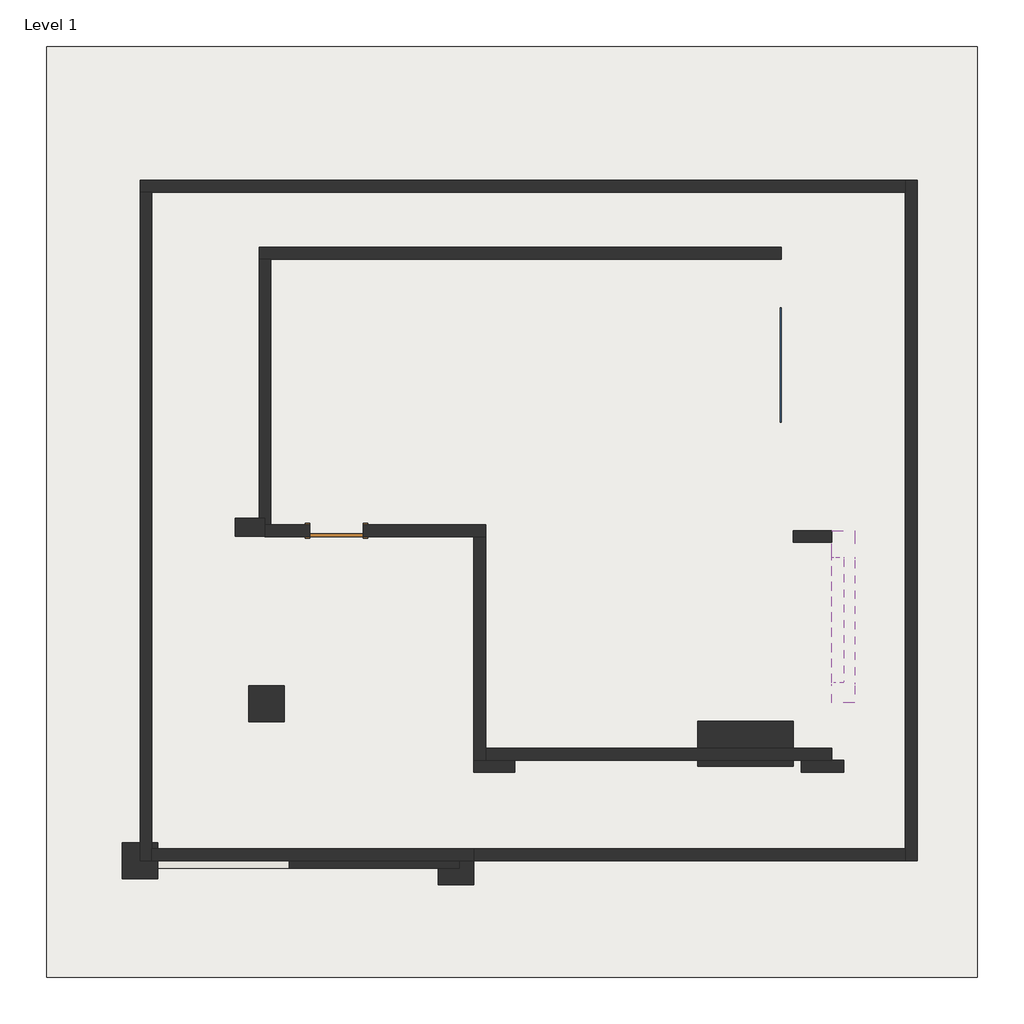
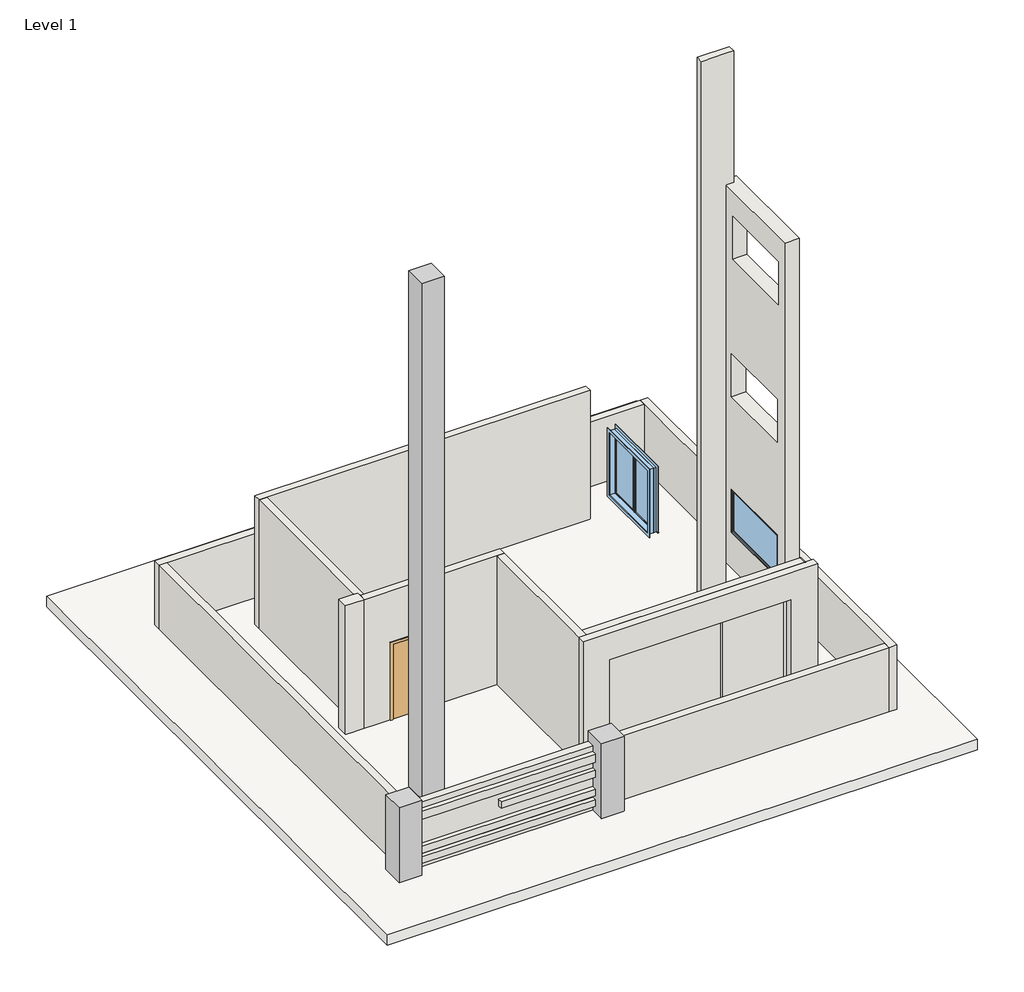
# One storey: 16 walls, 3 columns, 2 windows, 1 door, 1 slab.
"""IFC4 building model written with IfcOpenShell, lengths in millimetres."""

from ifc_helpers import new_model, si_unit, frame, origin, origin_with_axes, place, context, project, spatial, polyline, outline, extrude, faceted_brep, transform, mapped, element, save
from components import column_edfe3d85, door_54dd4da4, walls_2_walls_2_0b909519, walls_3_walls_3_385398a2, walls_4_walls_4_47acbb33, window_b085ff8d, window_a973ac2f

model = new_model("IFC4")

# Units and contexts
model_context = context("Model", 3, world=origin())
ifc_project = project(units=[si_unit("LENGTHUNIT", "METRE", prefix="MILLI")], contexts=[model_context])

# Site, building, storey
site = spatial("IfcSite", under=ifc_project)
building = spatial("IfcBuilding", under=site)
storey = spatial("IfcBuildingStorey", under=building, Name="Level 1", Elevation=0.0)

# Columns
placement = place(None, origin())
element("IfcColumn", 1, ObjectType="Rectangular Column : 24\" x 24\"", at=placement, inside=storey, context=model_context, shape_type="Brep", body=[
    faceted_brep([(-11835.7165692, -1.8724828, 2133.6), (-12445.3165692, -1.8724828, 2133.6), (-12445.3165692, -611.4724828, 2133.6), (-11835.7165692, -611.4724828, 2133.6), (-11937.3165692, -1.8724828, 0.0), (-11835.7165692, -1.8724828, 0.0), (-11835.7165692, -103.4724828, 0.0), (-11937.3165692, -103.4724828, 0.0), (-11937.3165692, -1.8724828, 1828.8), (-12140.5165692, -1.8724828, 1828.8), (-12140.5165692, -1.8724828, 0.0), (-12445.3165692, -1.8724828, 0.0), (-12445.3165692, -611.4724828, 0.0), (-11835.7165692, -611.4724828, 0.0), (-11835.7165692, -306.6724828, 0.0), (-11835.7165692, -306.6724828, 1828.8), (-11835.7165692, -103.4724828, 1828.8), (-11937.3165692, -103.4724828, 1828.8), (-12140.5165692, -306.6724828, 1828.8), (-12140.5165692, -306.6724828, 0.0), (-11937.3165692, -306.6724828, 1828.8), (-11937.3165692, -306.6724828, 0.0)], [[[0, 1, 2, 3]], [[4, 5, 6, 7]], [[1, 0, 5, 4, 8, 9, 10, 11]], [[2, 1, 11, 12]], [[3, 2, 12, 13]], [[0, 3, 13, 14, 15, 16, 6, 5]], [[8, 4, 7, 17]], [[18, 19, 10, 9]], [[20, 18, 9, 8, 17]], [[19, 18, 20, 21]], [[20, 15, 14, 21]], [[16, 17, 7, 6]], [[15, 20, 17, 16]], [[13, 12, 11, 10, 19, 21, 14]]]),
])
element("IfcColumn", 2, ObjectType="Rectangular Column : 24\" x 24\"", at=placement, inside=storey, context=model_context, shape_type="Brep", body=[
    faceted_brep([(-6456.5821198, -102.7094845, 2133.6), (-7066.1821198, -102.7094845, 2133.6), (-7066.1821198, -712.3094845, 2133.6), (-6456.5821198, -712.3094845, 2133.6), (-7066.1821198, -102.7094845, 0.0), (-6456.5821198, -102.7094845, 0.0), (-6456.5821198, -103.4724828, 0.0), (-7066.1821198, -103.4724828, 0.0), (-6456.5821198, -102.7094845, 1828.8), (-7066.1821198, -103.4724828, 1828.8), (-7066.1821198, -306.6724828, 1828.8), (-7066.1821198, -306.6724828, 0.0), (-7066.1821198, -712.3094845, 0.0), (-6456.5821198, -712.3094845, 0.0), (-6456.5821198, -306.6724828, 0.0), (-6456.5821198, -306.6724828, 1828.8), (-6456.5821198, -103.4724828, 1828.8)], [[[0, 1, 2, 3]], [[4, 5, 6, 7]], [[1, 0, 8, 5, 4]], [[2, 1, 4, 7, 9, 10, 11, 12]], [[3, 2, 12, 13]], [[0, 3, 13, 14, 15, 16, 6, 5, 8]], [[10, 15, 14, 11]], [[16, 9, 7, 6]], [[15, 10, 9, 16]], [[13, 12, 11, 14]]]),
])
column_shape = column_edfe3d85(model_context)
element("IfcColumn", 3, ObjectType="Rectangular Column : 24\" x 24\"", at=placement, inside=storey, context=model_context, shape_type="MappedRepresentation", body=[
    mapped(column_shape, transform((-9987.1821198, 2368.60098, 0.0), x_axis=(1.0, 0.0, 0.0), y_axis=(0.0, 1.0, 0.0), z_axis=(0.0, 0.0, 1.0))),
])

# Door
door_shape = door_54dd4da4(model_context)
element("IfcDoor", 4, ObjectType="Single-Flush : 36\" x 84\"", at=placement, inside=storey, context=model_context, shape_type="MappedRepresentation", body=[
    mapped(door_shape, transform((-8793.3821198, 5315.00098, 0.0), x_axis=(-1.0, 0.0, 0.0), y_axis=(0.0, -1.0, 0.0), z_axis=(0.0, 0.0, 1.0))),
])

# Slab
element("IfcSlab", 5, ObjectType="Generic - 12\"", at=placement, inside=storey, context=model_context, shape_type="SweptSolid", body=[
    extrude(outline(polyline([(2117.6840298, 13555.8620749), (2117.6840298, -2293.7379251), (-13731.9159702, -2293.7379251), (-13731.9159702, 13555.8620749), (2117.6840298, 13555.8620749)])), frame((0.0, 0.0, -304.8), z_axis=(0.0, 0.0, 1.0), x_axis=(1.0, 0.0, 0.0)), (0.0, 0.0, 1.0), 304.8),
])

# Walls
element("IfcWall", 6, ObjectType="Generic - 12\"", at=placement, inside=storey, context=model_context, shape_type="Brep", body=[
    faceted_brep([(-10520.5932957, 5216.0652184, 0.0), (-10012.5821198, 5216.0652184, 0.0), (-10012.5821198, 5216.0652184, 3657.6), (-10520.5932957, 5216.0652184, 3657.6), (-10520.5932957, 5520.8652184, 0.0), (-10520.5932957, 5520.8652184, 3657.6), (-10114.1821198, 5520.8652184, 3657.6), (-10012.5821198, 5520.8652184, 3657.6), (-10012.5821198, 5520.8652184, 0.0), (-10114.1821198, 5520.8652184, 0.0), (-10012.5821198, 5416.60098, 0.0), (-10012.5821198, 5416.60098, 3657.6)], [[[0, 1, 2, 3]], [[4, 5, 6, 7, 8, 9]], [[1, 0, 4, 9, 8, 10]], [[2, 1, 10, 8, 7, 11]], [[3, 2, 11, 7, 6, 5]], [[0, 3, 5, 4]]]),
])
element("IfcWall", 7, ObjectType="Generic - 8\"", at=placement, inside=storey, context=model_context, shape_type="Brep", body=[
    faceted_brep([(-10114.1821198, 9937.80098, 0.0), (-9910.9821198, 9937.80098, 0.0), (-1224.1821198, 9937.80098, 0.0), (-1224.1821198, 9937.80098, 3657.6), (-9910.9821198, 9937.80098, 3657.6), (-10114.1821198, 9937.80098, 3657.6), (-10114.1821198, 10141.00098, 0.0), (-10114.1821198, 10141.00098, 3657.6), (-1224.1821198, 10141.00098, 3657.6), (-1224.1821198, 10141.00098, 0.0)], [[[0, 1, 2, 3, 4, 5]], [[6, 7, 8, 9]], [[2, 1, 0, 6, 9]], [[0, 5, 7, 6]], [[5, 4, 3, 8, 7]], [[3, 2, 9, 8]]]),
])
element("IfcWall", 8, ObjectType="Generic - 8\"", at=placement, inside=storey, context=model_context, shape_type="SweptSolid", body=[
    extrude(outline(polyline([(-9910.9821198, 9937.80098), (-9910.9821198, 5416.60098), (-10012.5821198, 5416.60098), (-10012.5821198, 5520.8652184), (-10114.1821198, 5520.8652184), (-10114.1821198, 9937.80098), (-9910.9821198, 9937.80098)])), origin_with_axes(), (0.0, 0.0, 1.0), 3657.6),
])
element("IfcWall", 9, ObjectType="Generic - 8\"", at=placement, inside=storey, context=model_context, shape_type="SweptSolid", body=[
    extrude(outline(polyline([(0.0, -360.5821198), (3657.6, -360.5821198), (3657.6, -385.9821198), (3657.6, -6253.3821198), (0.0, -6253.3821198), (0.0, -360.5821198)])), frame((0.0, 1403.40098, 0.0), z_axis=(0.0, 1.0, 0.0), x_axis=(0.0, 0.0, 1.0)), (0.0, 0.0, 1.0), 203.2),
])
element("IfcWall", 10, ObjectType="Generic - 8\"", at=placement, inside=storey, context=model_context, shape_type="Brep", body=[
    faceted_brep([(-10012.5821198, 5213.40098, 0.0), (-9250.5821198, 5213.40098, 0.0), (-9250.5821198, 5213.40098, 2133.6), (-8336.1821198, 5213.40098, 2133.6), (-8336.1821198, 5213.40098, 0.0), (-6456.5821198, 5213.40098, 0.0), (-6253.3821198, 5213.40098, 0.0), (-6253.3821198, 5213.40098, 3657.6), (-6456.5821198, 5213.40098, 3657.6), (-10012.5821198, 5213.40098, 3657.6), (-9250.5821198, 5416.60098, 2133.6), (-9250.5821198, 5416.60098, 0.0), (-9910.9821198, 5416.60098, 0.0), (-10012.5821198, 5416.60098, 0.0), (-10012.5821198, 5416.60098, 3657.6), (-9910.9821198, 5416.60098, 3657.6), (-6253.3821198, 5416.60098, 3657.6), (-6253.3821198, 5416.60098, 0.0), (-8336.1821198, 5416.60098, 0.0), (-8336.1821198, 5416.60098, 2133.6), (-10012.5821198, 5216.0652184, 0.0), (-10012.5821198, 5216.0652184, 3657.6)], [[[0, 1, 2, 3, 4, 5, 6, 7, 8, 9]], [[10, 11, 12, 13, 14, 15, 16, 17, 18, 19]], [[18, 17, 6, 5, 4]], [[13, 12, 11, 1, 0, 20]], [[9, 8, 7, 16, 15, 14, 21]], [[0, 9, 21, 14, 13, 20]], [[7, 6, 17, 16]], [[2, 1, 11, 10]], [[3, 2, 10, 19]], [[4, 3, 19, 18]]]),
])
element("IfcWall", 11, ObjectType="Generic - 8\"", at=placement, inside=storey, context=model_context, shape_type="Brep", body=[
    faceted_brep([(-6456.5821198, 5213.40098, 0.0), (-6456.5821198, 1403.40098, 0.0), (-6456.5821198, 1403.40098, 3657.6), (-6456.5821198, 5213.40098, 3657.6), (-6253.3821198, 5213.40098, 0.0), (-6253.3821198, 5213.40098, 3657.6), (-6253.3821198, 1606.60098, 3657.6), (-6253.3821198, 1403.40098, 3657.6), (-6253.3821198, 1403.40098, 0.0), (-6253.3821198, 1606.60098, 0.0)], [[[0, 1, 2, 3]], [[4, 5, 6, 7, 8, 9]], [[1, 0, 4, 9, 8]], [[3, 2, 7, 6, 5]], [[0, 3, 5, 4]], [[2, 1, 8, 7]]]),
])
element("IfcWall", 12, ObjectType="Generic - 8\"", at=placement, inside=storey, context=model_context, shape_type="SweptSolid", body=[
    extrude(outline(polyline([(0.0, -6456.5821198), (0.0, -5759.4741466), (2895.6, -5759.4741466), (2895.6, -882.6741466), (0.0, -882.6741466), (0.0, -157.3821198), (3657.6, -157.3821198), (3657.6, -6456.5821198), (0.0, -6456.5821198)])), frame((0.0, 1200.20098, 0.0), z_axis=(0.0, 1.0, 0.0), x_axis=(0.0, 0.0, 1.0)), (0.0, 0.0, 1.0), 203.2),
])
element("IfcWall", 13, ObjectType="Generic - 8\"", at=placement, inside=storey, context=model_context, shape_type="Brep", body=[
    faceted_brep([(-1020.9821198, 5111.80098, 15849.6), (-1020.9821198, 5111.80098, 0.0), (-360.5821198, 5111.80098, 0.0), (-360.5821198, 5111.80098, 7315.2), (-157.3821198, 5111.80098, 7315.2), (-157.3821198, 5111.80098, 15849.6), (-360.5821198, 5111.80098, 15849.6), (-1020.9821198, 5315.00098, 0.0), (-1020.9821198, 5315.00098, 15849.6), (-157.3821198, 5315.00098, 15849.6), (-157.3821198, 5315.00098, 7315.2), (-360.5821198, 5315.00098, 7315.2), (-360.5821198, 5315.00098, 0.0)], [[[0, 1, 2, 3, 4, 5, 6]], [[7, 8, 9, 10, 11, 12]], [[2, 1, 7, 12]], [[0, 6, 5, 9, 8]], [[10, 4, 3, 11]], [[3, 2, 12, 11]], [[5, 4, 10, 9]], [[0, 8, 7, 1]]]),
])
element("IfcWall", 14, ObjectType="Generic - 8\"", at=placement, inside=storey, context=model_context, shape_type="Brep", body=[
    faceted_brep([(-12140.5165692, 11072.5275172, 0.0), (-11937.3165692, 11072.5275172, 0.0), (889.6834308, 11072.5275172, 0.0), (889.6834308, 11072.5275172, 1828.8), (-11937.3165692, 11072.5275172, 1828.8), (-12140.5165692, 11072.5275172, 1828.8), (-12140.5165692, 11275.7275172, 0.0), (-12140.5165692, 11275.7275172, 1828.8), (889.6834308, 11275.7275172, 1828.8), (889.6834308, 11275.7275172, 0.0)], [[[0, 1, 2, 3, 4, 5]], [[6, 7, 8, 9]], [[2, 1, 0, 6, 9]], [[5, 4, 3, 8, 7]], [[0, 5, 7, 6]], [[3, 2, 9, 8]]]),
])
element("IfcWall", 15, ObjectType="Generic - 8\"", at=placement, inside=storey, context=model_context, shape_type="Brep", body=[
    faceted_brep([(-11937.3165692, -306.6724828, 0.0), (-11937.3165692, -103.4724828, 0.0), (-11937.3165692, -1.8724828, 0.0), (-11937.3165692, 11072.5275172, 0.0), (-11937.3165692, 11072.5275172, 1828.8), (-11937.3165692, -1.8724828, 1828.8), (-11937.3165692, -103.4724828, 1828.8), (-11937.3165692, -306.6724828, 1828.8), (-12140.5165692, -306.6724828, 0.0), (-12140.5165692, -306.6724828, 1828.8), (-12140.5165692, -1.8724828, 1828.8), (-12140.5165692, 11072.5275172, 1828.8), (-12140.5165692, 11072.5275172, 0.0), (-12140.5165692, -1.8724828, 0.0)], [[[0, 1, 2, 3, 4, 5, 6, 7]], [[8, 9, 10, 11, 12, 13]], [[3, 2, 1, 0, 8, 13, 12]], [[7, 6, 5, 4, 11, 10, 9]], [[4, 3, 12, 11]], [[0, 7, 9, 8]]]),
])
element("IfcWall", 16, ObjectType="Generic - 8\"", at=placement, inside=storey, context=model_context, shape_type="Brep", body=[
    faceted_brep([(889.6834308, 11275.7275172, 0.0), (889.6834308, 11072.5275172, 0.0), (889.6834308, -102.7094845, 0.0), (889.6834308, -305.9094845, 0.0), (889.6834308, -305.9094845, 1828.8), (889.6834308, -102.7094845, 1828.8), (889.6834308, 11072.5275172, 1828.8), (889.6834308, 11275.7275172, 1828.8), (1092.8834308, 11275.7275172, 0.0), (1092.8834308, 11275.7275172, 1828.8), (1092.8834308, -305.9094845, 1828.8), (1092.8834308, -305.9094845, 0.0)], [[[0, 1, 2, 3, 4, 5, 6, 7]], [[8, 9, 10, 11]], [[3, 2, 1, 0, 8, 11]], [[7, 6, 5, 4, 10, 9]], [[0, 7, 9, 8]], [[4, 3, 11, 10]]]),
])
element("IfcWall", 17, ObjectType="Generic - 8\"", at=placement, inside=storey, context=model_context, shape_type="Brep", body=[
    faceted_brep([(889.6834308, -102.7094845, 0.0), (-6456.5821198, -102.7094845, 0.0), (-6456.5821198, -102.7094845, 1828.8), (889.6834308, -102.7094845, 1828.8), (889.6834308, -305.9094845, 0.0), (889.6834308, -305.9094845, 1828.8), (-6456.5821198, -305.9094845, 1828.8), (-6456.5821198, -305.9094845, 0.0), (-6456.5821198, -103.4724828, 0.0), (-6456.5821198, -103.4724828, 1828.8)], [[[0, 1, 2, 3]], [[4, 5, 6, 7]], [[1, 0, 4, 7, 8]], [[2, 1, 8, 7, 6, 9]], [[3, 2, 9, 6, 5]], [[0, 3, 5, 4]]]),
])
element("IfcWall", 18, ObjectType="Generic - 8\"", at=placement, inside=storey, context=model_context, shape_type="Brep", body=[
    faceted_brep([(-11937.3165692, -306.6724828, 0.0), (-11835.7165692, -306.6724828, 0.0), (-7066.1821198, -306.6724828, 0.0), (-6456.5821198, -306.6724828, 0.0), (-6456.5821198, -306.6724828, 1828.8), (-7066.1821198, -306.6724828, 1828.8), (-11835.7165692, -306.6724828, 1828.8), (-11937.3165692, -306.6724828, 1828.8), (-11937.3165692, -103.4724828, 0.0), (-11937.3165692, -103.4724828, 1828.8), (-11835.7165692, -103.4724828, 1828.8), (-7066.1821198, -103.4724828, 1828.8), (-6456.5821198, -103.4724828, 1828.8), (-6456.5821198, -103.4724828, 0.0), (-7066.1821198, -103.4724828, 0.0), (-11835.7165692, -103.4724828, 0.0), (-6456.5821198, -305.9094845, 0.0), (-6456.5821198, -305.9094845, 1828.8)], [[[0, 1, 2, 3, 4, 5, 6, 7]], [[8, 9, 10, 11, 12, 13, 14, 15]], [[3, 2, 1, 0, 8, 15, 14, 13, 16]], [[4, 3, 16, 13, 12, 17]], [[7, 6, 5, 4, 17, 12, 11, 10, 9]], [[0, 7, 9, 8]]]),
])
walls_2_walls_2_shape = walls_2_walls_2_0b909519(model_context)
element("IfcWall", 19, ObjectType="Walls 2 : Walls 2", at=placement, inside=storey, context=model_context, shape_type="MappedRepresentation", body=[
    mapped(walls_2_walls_2_shape, transform((0.0, 0.0, 0.0), x_axis=(1.0, 0.0, 0.0), y_axis=(0.0, 1.0, 0.0), z_axis=(0.0, 0.0, 1.0))),
])
walls_3_walls_3_shape = walls_3_walls_3_385398a2(model_context)
element("IfcWall", 20, ObjectType="Walls 3 : Walls 3", at=placement, inside=storey, context=model_context, shape_type="MappedRepresentation", body=[
    mapped(walls_3_walls_3_shape, transform((0.0, 0.0, 0.0), x_axis=(1.0, 0.0, 0.0), y_axis=(0.0, 1.0, 0.0), z_axis=(0.0, 0.0, 1.0))),
])
walls_4_walls_4_shape = walls_4_walls_4_47acbb33(model_context)
element("IfcWall", 21, ObjectType="Walls 4 : Walls 4", at=placement, inside=storey, context=model_context, shape_type="MappedRepresentation", body=[
    mapped(walls_4_walls_4_shape, transform((0.0, 0.0, 0.0), x_axis=(1.0, 0.0, 0.0), y_axis=(0.0, 1.0, 0.0), z_axis=(0.0, 0.0, 1.0))),
])

# Windows
window_shape = window_b085ff8d(model_context)
element("IfcWindow", 22, ObjectType="Casement Dbl with Trim : 72\" x 36\"", at=placement, inside=storey, context=model_context, shape_type="MappedRepresentation", body=[
    mapped(window_shape, transform((-1141.6321198, 8134.40098, 0.0), x_axis=(0.0, -1.0, 0.0), y_axis=(1.0, 0.0, 0.0), z_axis=(0.0, 0.0, 1.0))),
])
window_2_shape = window_a973ac2f(model_context)
element("IfcWindow", 23, ObjectType="Fixed : 36\" x 72\"", at=placement, inside=storey, context=model_context, shape_type="MappedRepresentation", body=[
    mapped(window_2_shape, transform((-258.9821198, 3829.10098, 2100.7438024), x_axis=(0.0, 1.0, 0.0), y_axis=(-1.0, 0.0, 0.0), z_axis=(0.0, 0.0, 1.0))),
])

save(model, "model.ifc")

# Revit data of these elements
# Type "Rectangular Column : 24\" x 24\""
#   Assembly Code = "B1010200"
#   Depth = 2' - 0"
#   Offset Base = 0' - 0"
#   Offset Top = 0' - 0"
#   Width = 2' - 0"
#   Material = none
# Type "Single-Flush : 36\" x 84\""
#   Type Mark = "1"
#   Construction Type Id = "MDOOR"
#   Assembly Code = "C1020"
#   Analytic Construction = "Metal"
#   Thickness = 0' - 2"
#   Heat Transfer Coefficient (U) = 0.651978 BTU/(h·ft²·°F)
#   Height = 7' - 0"
#   Trim Projection Ext = 0' - 1"
#   Trim Projection Int = 0' - 1"
#   Trim Width = 0' - 3"
#   Width = 3' - 0"
#   Define Thermal Properties by = 1
#   Door Material = Door - Panel
#   Frame Material = Door - Frame
#   Visual Light Transmittance = 0
#   Solar Heat Gain Coefficient = 0
#   Function = (empty or 0)
#   Wall Closure = (empty or 0)
# Type "Generic - 12\""
#   Assembly Code = "B1010"
#   Function = 0
#   Layers, outside or top first: 1' - 0" no material (function 1)
# Type "Generic - 12\""
#   Assembly Code = "B2010"
#   Layers, outside or top first: 1' - 0" no material (function 1)
# Type "Generic - 8\""
#   Assembly Code = "B2010"
#   Layers, outside or top first: 0' - 8" no material (function 1)
# Type "Casement Dbl with Trim : 72\" x 36\""
#   Type Mark = "11"
#   Construction Type Id = "GSP4R"
#   Assembly Code = "B2020100"
#   Analytic Construction = "1/8 in Pilkington single glazing"
#   Visual Light Transmittance = 0.9
#   Solar Heat Gain Coefficient = 0.78
#   Heat Transfer Coefficient (U) = 0.6496 BTU/(h·ft²·°F)
#   Height = 6' - 0"
#   Default Sill Height = 4' - 0"
#   Trim Projection - Ext. = 0' - 0 1/2"
#   Trim Projection - Int. = 0' - 0 3/4"
#   Trim Width - Exterior = 0' - 3 1/2"
#   Trim Width - Interior = 0' - 3 1/2"
#   Width = 6' - 0"
#   Window Inset = 0' - 0 3/4"
#   Define Thermal Properties by = 1
#   Glass Pane Material = Glass
#   Sash Material = Sash
#   Trim Exterior Material = Trim
#   Trim Interior Material = Trim
#   Wall Closure = (empty or 0)
# Type "Fixed : 36\" x 72\""
#   Type Mark = "9"
#   Construction Type Id = "GSP4R"
#   Assembly Code = "B2020100"
#   Analytic Construction = "1/8 in Pilkington single glazing"
#   Visual Light Transmittance = 0.9
#   Solar Heat Gain Coefficient = 0.78
#   Heat Transfer Coefficient (U) = 0.6496 BTU/(h·ft²·°F)
#   Height = 4' - 0"
#   Default Sill Height = 1' - 0"
#   Width = 7' - 0"
#   Window Inset = 0' - 0 3/4"
#   Define Thermal Properties by = 1
#   Glass Pane Material = Glass
#   Sash Material = Sash
#   Wall Closure = (empty or 0)
# Elements 1, 2 (IfcColumn, "Rectangular Column : 24\" x 24\"")
#   Phase Created = New Construction
#   Materials on its faces: "Default Wall"
# Element 3 (IfcColumn, "Rectangular Column : 24\" x 24\"")
#   Phase Created = New Construction
# Element 4 (IfcDoor, "Single-Flush : 36\" x 84\"")
#   Phase Created = New Construction
#   Materials on its faces: "Door - Frame", "Door - Panel"
# Element 5 (IfcSlab, "Generic - 12\"")
#   Height Offset From Level = 0' - 0"
#   Phase Created = New Construction
#   Materials on its faces: "Default Floor"
# Element 6 (IfcWall, "Generic - 12\"")
#   Top Offset = 0' - 0"
#   Base Offset = 0' - 0"
#   Unconnected Height = 12' - 0"
#   wall height = 12' - 0"
#   Phase Created = New Construction
#   Base Constraint = Level 1
#   Materials on its faces: "Default Wall"
# Elements 7, 8, 10 (IfcWall, "Generic - 8\"")
#   Top Offset = 0' - 0"
#   Base Offset = 0' - 0"
#   Unconnected Height = 12' - 0"
#   wall height = 12' - 0"
#   Phase Created = New Construction
#   Base Constraint = Level 1
#   Materials on its faces: "Default Wall"
# Elements 9, 11, 12 (IfcWall, "Generic - 8\"")
#   Top Offset = 0' - 0"
#   Base Offset = 0' - 0"
#   Unconnected Height = 12' - 0"
#   wall height = 12' - 0"
#   Phase Created = New Construction
#   Base Constraint = Level 1
#   Materials on its faces: "Default Wall", "Laminate, Ivory, Matte"
# Element 13 (IfcWall, "Generic - 8\"")
#   Top Offset = 0' - 0"
#   Base Offset = 0' - 0"
#   Unconnected Height = 52' - 0"
#   wall height = 52' - 0"
#   Phase Created = New Construction
#   Base Constraint = Level 1
#   Materials on its faces: "Default Wall"
# Elements 14, 15, 16, 17, 18 (IfcWall, "Generic - 8\"")
#   Top Offset = 0' - 0"
#   Base Offset = 0' - 0"
#   Unconnected Height = 6' - 0"
#   wall height = 6' - 0"
#   Phase Created = New Construction
#   Base Constraint = Level 1
#   Materials on its faces: "Default Wall"
# Element 19 (IfcWall, "Walls 2 : Walls 2")
#   Phase Created = New Construction
#   Materials on its faces: "Default Wall"
# Element 20 (IfcWall, "Walls 3 : Walls 3")
#   Phase Created = New Construction
#   Materials on its faces: "Default Wall"
# Element 21 (IfcWall, "Walls 4 : Walls 4")
#   Phase Created = New Construction
#   Materials on its faces: "Default Wall"
# Element 22 (IfcWindow, "Casement Dbl with Trim : 72\" x 36\"")
#   Mark = "10"
#   Phase Created = New Construction
#   Materials on its faces: "Sash", "Trim", "Glass"
# Element 23 (IfcWindow, "Fixed : 36\" x 72\"")
#   Mark = "5"
#   Phase Created = New Construction
#   Materials on its faces: "Sash", "Glass"
# Materials
#   "Door - Panel": class "Wood", colour RGB 210 159 95, transparency 0
#   "Door - Frame": colour RGB 118 70 51, transparency 0
#   "Glass": class "Glass", colour RGB 0 128 192, transparency 0.75, Description = "Soda Lime Glass", Cost = 0
#   "Sash": class "Wood", colour RGB 224 178 126, transparency 0
#   "Trim": class "Wood", colour RGB 224 178 126, transparency 0
#   "Default Wall": colour RGB 128 128 128, transparency 0
#   "Default Floor": colour RGB 128 128 128, transparency 0
#   "Laminate, Ivory, Matte": class "Plastic", colour RGB 247 247 239, transparency 0, Description = "Plastic Laminate - Ivory, Matte", Cost = 0
